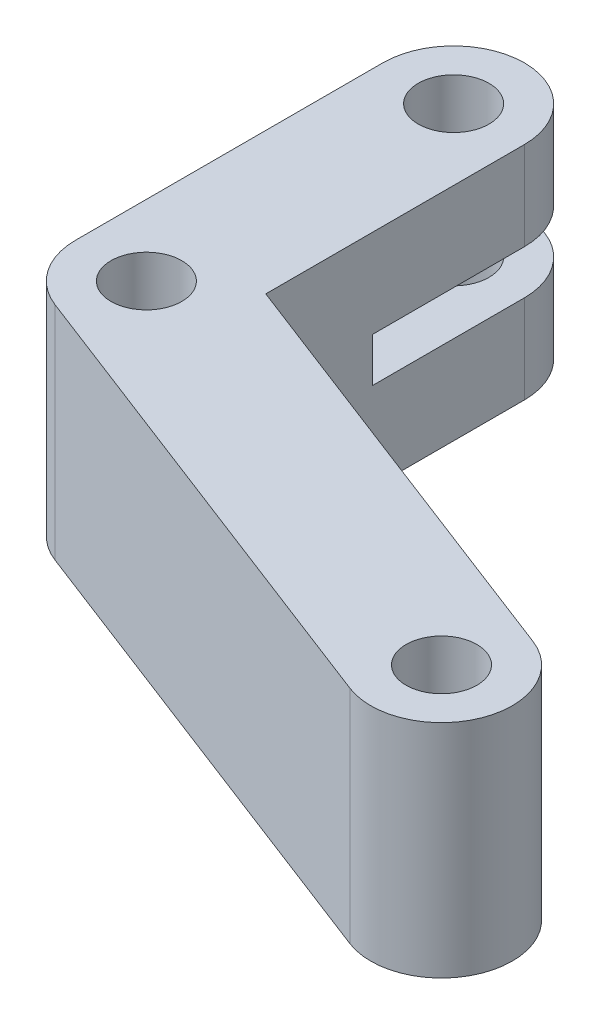
ISO-10303-21;
HEADER;
FILE_DESCRIPTION(('STEP AP214'),'2;1');
FILE_NAME('part.step','',(''),(''),'','','');
FILE_SCHEMA(('AUTOMOTIVE_DESIGN { 1 0 10303 214 1 1 1 1 }'));
ENDSEC;
DATA;
#1=APPLICATION_CONTEXT('core data for automotive mechanical design processes');
#2=APPLICATION_PROTOCOL_DEFINITION('international standard','automotive_design',2000,#1);
#3=PRODUCT_CONTEXT('',#1,'mechanical');
#4=PRODUCT('Part','Part','',(#3));
#5=PRODUCT_RELATED_PRODUCT_CATEGORY('part','',(#4));
#6=PRODUCT_DEFINITION_FORMATION('','',#4);
#7=PRODUCT_DEFINITION_CONTEXT('part definition',#1,'design');
#8=PRODUCT_DEFINITION('design','',#6,#7);
#9=PRODUCT_DEFINITION_SHAPE('','',#8);
#10=(LENGTH_UNIT() NAMED_UNIT(*) SI_UNIT(.MILLI.,.METRE.));
#11=(NAMED_UNIT(*) PLANE_ANGLE_UNIT() SI_UNIT($,.RADIAN.));
#12=(NAMED_UNIT(*) SI_UNIT($,.STERADIAN.) SOLID_ANGLE_UNIT());
#13=UNCERTAINTY_MEASURE_WITH_UNIT(LENGTH_MEASURE(1.E-05),#10,'distance_accuracy_value','');
#14=(GEOMETRIC_REPRESENTATION_CONTEXT(3) GLOBAL_UNCERTAINTY_ASSIGNED_CONTEXT((#13)) GLOBAL_UNIT_ASSIGNED_CONTEXT((#10,
#11,#12)) REPRESENTATION_CONTEXT('',''));
#15=CARTESIAN_POINT('',(0.,0.,0.));
#16=DIRECTION('',(0.,0.,1.));
#17=DIRECTION('',(1.,0.,0.));
#18=AXIS2_PLACEMENT_3D('',#15,#16,#17);
#19=CARTESIAN_POINT('',(0.,25.,-34.72));
#20=DIRECTION('',(0.,-1.,0.));
#21=DIRECTION('',(0.,0.,-1.));
#22=AXIS2_PLACEMENT_3D('',#19,#20,#21);
#23=CYLINDRICAL_SURFACE('',#22,8.);
#24=CARTESIAN_POINT('',(0.,10.,-34.72));
#25=DIRECTION('',(0.,-1.,0.));
#26=DIRECTION('',(0.,0.,-1.));
#27=AXIS2_PLACEMENT_3D('',#24,#25,#26);
#28=CIRCLE('',#27,8.);
#29=CARTESIAN_POINT('',(-8.,10.,-34.72));
#30=VERTEX_POINT('',#29);
#31=CARTESIAN_POINT('',(8.,10.,-34.72));
#32=VERTEX_POINT('',#31);
#33=EDGE_CURVE('E184',#30,#32,#28,.T.);
#34=ORIENTED_EDGE('',*,*,#33,.T.);
#35=DIRECTION('',(0.,-1.,0.));
#36=VECTOR('',#35,1.);
#37=CARTESIAN_POINT('',(8.,25.,-34.72));
#38=LINE('',#37,#36);
#39=CARTESIAN_POINT('',(8.,0.,-34.72));
#40=VERTEX_POINT('',#39);
#41=EDGE_CURVE('E96',#32,#40,#38,.T.);
#42=ORIENTED_EDGE('',*,*,#41,.T.);
#43=CARTESIAN_POINT('',(0.,0.,-34.72));
#44=DIRECTION('',(0.,1.,0.));
#45=DIRECTION('',(0.,0.,1.));
#46=AXIS2_PLACEMENT_3D('',#43,#44,#45);
#47=CIRCLE('',#46,8.);
#48=CARTESIAN_POINT('',(-8.00000000000001,0.,-34.72));
#49=VERTEX_POINT('',#48);
#50=EDGE_CURVE('E144',#40,#49,#47,.T.);
#51=ORIENTED_EDGE('',*,*,#50,.T.);
#52=DIRECTION('',(0.,-1.,0.));
#53=VECTOR('',#52,1.);
#54=CARTESIAN_POINT('',(-8.00000000000001,25.,-34.72));
#55=LINE('',#54,#53);
#56=EDGE_CURVE('E171',#30,#49,#55,.T.);
#57=ORIENTED_EDGE('',*,*,#56,.F.);
#58=EDGE_LOOP('',(#34,#42,#51,#57));
#59=FACE_BOUND('',#58,.T.);
#60=ADVANCED_FACE('F41',(#59),#23,.T.);
#61=CARTESIAN_POINT('',(0.,0.,-34.72));
#62=DIRECTION('',(0.,1.,0.));
#63=DIRECTION('',(0.,0.,1.));
#64=AXIS2_PLACEMENT_3D('',#61,#62,#63);
#65=CYLINDRICAL_SURFACE('',#64,4.);
#66=CARTESIAN_POINT('',(0.,10.,-34.72));
#67=DIRECTION('',(0.,-1.,0.));
#68=DIRECTION('',(0.,0.,-1.));
#69=AXIS2_PLACEMENT_3D('',#66,#67,#68);
#70=CIRCLE('',#69,4.);
#71=CARTESIAN_POINT('',(0.,10.,-38.72));
#72=VERTEX_POINT('',#71);
#73=EDGE_CURVE('E180',#72,#72,#70,.F.);
#74=ORIENTED_EDGE('',*,*,#73,.T.);
#75=EDGE_LOOP('',(#74));
#76=FACE_BOUND('',#75,.T.);
#77=CARTESIAN_POINT('',(0.,0.,-34.72));
#78=DIRECTION('',(0.,1.,0.));
#79=DIRECTION('',(0.,0.,1.));
#80=AXIS2_PLACEMENT_3D('',#77,#78,#79);
#81=CIRCLE('',#80,4.);
#82=CARTESIAN_POINT('',(0.,0.,-30.72));
#83=VERTEX_POINT('',#82);
#84=EDGE_CURVE('E146',#83,#83,#81,.T.);
#85=ORIENTED_EDGE('',*,*,#84,.F.);
#86=EDGE_LOOP('',(#85));
#87=FACE_BOUND('',#86,.T.);
#88=ADVANCED_FACE('F257',(#76,#87),#65,.F.);
#89=CARTESIAN_POINT('',(8.,25.,-34.72));
#90=VERTEX_POINT('',#89);
#91=CARTESIAN_POINT('',(8.,15.,-34.72));
#92=VERTEX_POINT('',#91);
#93=EDGE_CURVE('E159',#90,#92,#38,.T.);
#94=ORIENTED_EDGE('',*,*,#93,.T.);
#95=CARTESIAN_POINT('',(0.,15.,-34.72));
#96=DIRECTION('',(0.,1.,0.));
#97=DIRECTION('',(0.,0.,1.));
#98=AXIS2_PLACEMENT_3D('',#95,#96,#97);
#99=CIRCLE('',#98,8.);
#100=CARTESIAN_POINT('',(-8.,15.,-34.72));
#101=VERTEX_POINT('',#100);
#102=EDGE_CURVE('E57',#92,#101,#99,.T.);
#103=ORIENTED_EDGE('',*,*,#102,.T.);
#104=CARTESIAN_POINT('',(-8.00000000000001,25.,-34.72));
#105=VERTEX_POINT('',#104);
#106=EDGE_CURVE('E47',#105,#101,#55,.T.);
#107=ORIENTED_EDGE('',*,*,#106,.F.);
#108=CARTESIAN_POINT('',(0.,25.,-34.72));
#109=DIRECTION('',(0.,1.,0.));
#110=DIRECTION('',(0.,0.,1.));
#111=AXIS2_PLACEMENT_3D('',#108,#109,#110);
#112=CIRCLE('',#111,8.);
#113=EDGE_CURVE('E157',#90,#105,#112,.T.);
#114=ORIENTED_EDGE('',*,*,#113,.F.);
#115=EDGE_LOOP('',(#94,#103,#107,#114));
#116=FACE_BOUND('',#115,.T.);
#117=ADVANCED_FACE('F43',(#116),#23,.T.);
#118=CARTESIAN_POINT('',(-8.00000000000001,25.,-34.72));
#119=DIRECTION('',(1.,0.,0.));
#120=DIRECTION('',(0.,0.,-1.));
#121=AXIS2_PLACEMENT_3D('',#118,#119,#120);
#122=PLANE('',#121);
#123=DIRECTION('',(0.,-1.,0.));
#124=VECTOR('',#123,1.);
#125=CARTESIAN_POINT('',(-8.,25.,-17.57));
#126=LINE('',#125,#124);
#127=CARTESIAN_POINT('',(-8.,15.,-17.57));
#128=VERTEX_POINT('',#127);
#129=CARTESIAN_POINT('',(-8.,10.,-17.57));
#130=VERTEX_POINT('',#129);
#131=EDGE_CURVE('E197',#128,#130,#126,.T.);
#132=ORIENTED_EDGE('',*,*,#131,.T.);
#133=DIRECTION('',(0.,0.,-1.));
#134=VECTOR('',#133,1.);
#135=CARTESIAN_POINT('',(-8.00000000000001,10.,-34.72));
#136=LINE('',#135,#134);
#137=EDGE_CURVE('E192',#130,#30,#136,.T.);
#138=ORIENTED_EDGE('',*,*,#137,.T.);
#139=ORIENTED_EDGE('',*,*,#56,.T.);
#140=DIRECTION('',(0.,0.,1.));
#141=VECTOR('',#140,1.);
#142=CARTESIAN_POINT('',(-8.00000000000001,0.,-34.72));
#143=LINE('',#142,#141);
#144=CARTESIAN_POINT('',(-8.,0.,0.));
#145=VERTEX_POINT('',#144);
#146=EDGE_CURVE('E150',#49,#145,#143,.T.);
#147=ORIENTED_EDGE('',*,*,#146,.T.);
#148=DIRECTION('',(0.,-1.,0.));
#149=VECTOR('',#148,1.);
#150=CARTESIAN_POINT('',(-8.,25.,0.));
#151=LINE('',#150,#149);
#152=CARTESIAN_POINT('',(-8.,25.,0.));
#153=VERTEX_POINT('',#152);
#154=EDGE_CURVE('E169',#153,#145,#151,.T.);
#155=ORIENTED_EDGE('',*,*,#154,.F.);
#156=DIRECTION('',(0.,0.,1.));
#157=VECTOR('',#156,1.);
#158=CARTESIAN_POINT('',(-8.00000000000001,25.,-34.72));
#159=LINE('',#158,#157);
#160=EDGE_CURVE('E104',#105,#153,#159,.T.);
#161=ORIENTED_EDGE('',*,*,#160,.F.);
#162=ORIENTED_EDGE('',*,*,#106,.T.);
#163=DIRECTION('',(0.,0.,1.));
#164=VECTOR('',#163,1.);
#165=CARTESIAN_POINT('',(-8.00000000000001,15.,-34.72));
#166=LINE('',#165,#164);
#167=EDGE_CURVE('E179',#101,#128,#166,.T.);
#168=ORIENTED_EDGE('',*,*,#167,.T.);
#169=EDGE_LOOP('',(#132,#138,#139,#147,#155,#161,#162,#168));
#170=FACE_BOUND('',#169,.T.);
#171=ADVANCED_FACE('F240',(#170),#122,.F.);
#172=CARTESIAN_POINT('',(0.,25.,0.));
#173=DIRECTION('',(0.,-1.,0.));
#174=DIRECTION('',(0.,0.,-1.));
#175=AXIS2_PLACEMENT_3D('',#172,#173,#174);
#176=CYLINDRICAL_SURFACE('',#175,8.);
#177=CARTESIAN_POINT('',(0.,0.,0.));
#178=DIRECTION('',(0.,1.,0.));
#179=DIRECTION('',(0.,0.,1.));
#180=AXIS2_PLACEMENT_3D('',#177,#178,#179);
#181=CIRCLE('',#180,8.);
#182=CARTESIAN_POINT('',(-2.87524489022323,0.,7.46545154838239));
#183=VERTEX_POINT('',#182);
#184=EDGE_CURVE('E147',#145,#183,#181,.T.);
#185=ORIENTED_EDGE('',*,*,#184,.T.);
#186=DIRECTION('',(0.,-1.,0.));
#187=VECTOR('',#186,1.);
#188=CARTESIAN_POINT('',(-2.87524489022323,25.,7.46545154838239));
#189=LINE('',#188,#187);
#190=CARTESIAN_POINT('',(-2.87524489022323,25.,7.46545154838239));
#191=VERTEX_POINT('',#190);
#192=EDGE_CURVE('E164',#191,#183,#189,.T.);
#193=ORIENTED_EDGE('',*,*,#192,.F.);
#194=CARTESIAN_POINT('',(0.,25.,0.));
#195=DIRECTION('',(0.,1.,0.));
#196=DIRECTION('',(0.,0.,1.));
#197=AXIS2_PLACEMENT_3D('',#194,#195,#196);
#198=CIRCLE('',#197,8.);
#199=EDGE_CURVE('E217',#153,#191,#198,.T.);
#200=ORIENTED_EDGE('',*,*,#199,.F.);
#201=ORIENTED_EDGE('',*,*,#154,.T.);
#202=EDGE_LOOP('',(#185,#193,#200,#201));
#203=FACE_BOUND('',#202,.T.);
#204=ADVANCED_FACE('F225',(#203),#176,.T.);
#205=CARTESIAN_POINT('',(-2.87524489022323,25.,7.46545154838239));
#206=DIRECTION('',(0.359405611277904,0.,-0.9331814435478));
#207=DIRECTION('',(-0.9331814435478,0.,-0.359405611277904));
#208=AXIS2_PLACEMENT_3D('',#205,#206,#207);
#209=PLANE('',#208);
#210=DIRECTION('',(0.9331814435478,0.,0.359405611277904));
#211=VECTOR('',#210,1.);
#212=CARTESIAN_POINT('',(-2.87524489022323,0.,7.46545154838239));
#213=LINE('',#212,#211);
#214=CARTESIAN_POINT('',(51.3647551097768,0.,28.3554515483825));
#215=VERTEX_POINT('',#214);
#216=EDGE_CURVE('E155',#183,#215,#213,.T.);
#217=ORIENTED_EDGE('',*,*,#216,.T.);
#218=DIRECTION('',(0.,-1.,0.));
#219=VECTOR('',#218,1.);
#220=CARTESIAN_POINT('',(51.3647551097768,25.,28.3554515483825));
#221=LINE('',#220,#219);
#222=CARTESIAN_POINT('',(51.3647551097768,25.,28.3554515483825));
#223=VERTEX_POINT('',#222);
#224=EDGE_CURVE('E136',#223,#215,#221,.T.);
#225=ORIENTED_EDGE('',*,*,#224,.F.);
#226=DIRECTION('',(0.9331814435478,0.,0.359405611277904));
#227=VECTOR('',#226,1.);
#228=CARTESIAN_POINT('',(-2.87524489022323,25.,7.46545154838239));
#229=LINE('',#228,#227);
#230=EDGE_CURVE('E122',#191,#223,#229,.T.);
#231=ORIENTED_EDGE('',*,*,#230,.F.);
#232=ORIENTED_EDGE('',*,*,#192,.T.);
#233=EDGE_LOOP('',(#217,#225,#231,#232));
#234=FACE_BOUND('',#233,.T.);
#235=ADVANCED_FACE('F226',(#234),#209,.F.);
#236=CARTESIAN_POINT('',(54.24,25.,20.89));
#237=DIRECTION('',(0.,-1.,0.));
#238=DIRECTION('',(0.,0.,-1.));
#239=AXIS2_PLACEMENT_3D('',#236,#237,#238);
#240=CYLINDRICAL_SURFACE('',#239,8.00000000000006);
#241=CARTESIAN_POINT('',(54.24,0.,20.89));
#242=DIRECTION('',(0.,1.,0.));
#243=DIRECTION('',(0.,0.,1.));
#244=AXIS2_PLACEMENT_3D('',#241,#242,#243);
#245=CIRCLE('',#244,8.00000000000006);
#246=CARTESIAN_POINT('',(57.1152448902233,0.,13.4245484516175));
#247=VERTEX_POINT('',#246);
#248=EDGE_CURVE('E134',#215,#247,#245,.T.);
#249=ORIENTED_EDGE('',*,*,#248,.T.);
#250=DIRECTION('',(0.,-1.,0.));
#251=VECTOR('',#250,1.);
#252=CARTESIAN_POINT('',(57.1152448902233,25.,13.4245484516175));
#253=LINE('',#252,#251);
#254=CARTESIAN_POINT('',(57.1152448902233,25.,13.4245484516175));
#255=VERTEX_POINT('',#254);
#256=EDGE_CURVE('E128',#255,#247,#253,.T.);
#257=ORIENTED_EDGE('',*,*,#256,.F.);
#258=CARTESIAN_POINT('',(54.24,25.,20.89));
#259=DIRECTION('',(0.,1.,0.));
#260=DIRECTION('',(0.,0.,1.));
#261=AXIS2_PLACEMENT_3D('',#258,#259,#260);
#262=CIRCLE('',#261,8.00000000000006);
#263=EDGE_CURVE('E117',#223,#255,#262,.T.);
#264=ORIENTED_EDGE('',*,*,#263,.F.);
#265=ORIENTED_EDGE('',*,*,#224,.T.);
#266=EDGE_LOOP('',(#249,#257,#264,#265));
#267=FACE_BOUND('',#266,.T.);
#268=ADVANCED_FACE('F131',(#267),#240,.T.);
#269=CARTESIAN_POINT('',(8.,25.,-5.49170276071211));
#270=DIRECTION('',(-0.359405611277902,0.,0.933181443547801));
#271=DIRECTION('',(0.933181443547801,0.,0.359405611277902));
#272=AXIS2_PLACEMENT_3D('',#269,#270,#271);
#273=PLANE('',#272);
#274=DIRECTION('',(-0.933181443547801,0.,-0.359405611277902));
#275=VECTOR('',#274,1.);
#276=CARTESIAN_POINT('',(8.,0.,-5.49170276071211));
#277=LINE('',#276,#275);
#278=CARTESIAN_POINT('',(8.,0.,-5.49170276071211));
#279=VERTEX_POINT('',#278);
#280=EDGE_CURVE('E154',#247,#279,#277,.T.);
#281=ORIENTED_EDGE('',*,*,#280,.T.);
#282=DIRECTION('',(0.,-1.,0.));
#283=VECTOR('',#282,1.);
#284=CARTESIAN_POINT('',(8.,25.,-5.49170276071211));
#285=LINE('',#284,#283);
#286=CARTESIAN_POINT('',(8.,25.,-5.49170276071211));
#287=VERTEX_POINT('',#286);
#288=EDGE_CURVE('E140',#287,#279,#285,.T.);
#289=ORIENTED_EDGE('',*,*,#288,.F.);
#290=DIRECTION('',(-0.933181443547801,0.,-0.359405611277902));
#291=VECTOR('',#290,1.);
#292=CARTESIAN_POINT('',(8.,25.,-5.49170276071211));
#293=LINE('',#292,#291);
#294=EDGE_CURVE('E121',#255,#287,#293,.T.);
#295=ORIENTED_EDGE('',*,*,#294,.F.);
#296=ORIENTED_EDGE('',*,*,#256,.T.);
#297=EDGE_LOOP('',(#281,#289,#295,#296));
#298=FACE_BOUND('',#297,.T.);
#299=ADVANCED_FACE('F137',(#298),#273,.F.);
#300=CARTESIAN_POINT('',(8.,25.,-34.72));
#301=DIRECTION('',(-1.,0.,0.));
#302=DIRECTION('',(0.,0.,1.));
#303=AXIS2_PLACEMENT_3D('',#300,#301,#302);
#304=PLANE('',#303);
#305=ORIENTED_EDGE('',*,*,#41,.F.);
#306=DIRECTION('',(0.,0.,1.));
#307=VECTOR('',#306,1.);
#308=CARTESIAN_POINT('',(8.,10.,-34.72));
#309=LINE('',#308,#307);
#310=CARTESIAN_POINT('',(8.,10.,-17.57));
#311=VERTEX_POINT('',#310);
#312=EDGE_CURVE('E177',#32,#311,#309,.T.);
#313=ORIENTED_EDGE('',*,*,#312,.T.);
#314=DIRECTION('',(0.,1.,0.));
#315=VECTOR('',#314,1.);
#316=CARTESIAN_POINT('',(8.,25.,-17.57));
#317=LINE('',#316,#315);
#318=CARTESIAN_POINT('',(8.,15.,-17.57));
#319=VERTEX_POINT('',#318);
#320=EDGE_CURVE('E11',#311,#319,#317,.T.);
#321=ORIENTED_EDGE('',*,*,#320,.T.);
#322=DIRECTION('',(0.,0.,-1.));
#323=VECTOR('',#322,1.);
#324=CARTESIAN_POINT('',(8.,15.,-34.72));
#325=LINE('',#324,#323);
#326=EDGE_CURVE('E175',#319,#92,#325,.T.);
#327=ORIENTED_EDGE('',*,*,#326,.T.);
#328=ORIENTED_EDGE('',*,*,#93,.F.);
#329=DIRECTION('',(0.,0.,-1.));
#330=VECTOR('',#329,1.);
#331=CARTESIAN_POINT('',(8.,25.,-34.72));
#332=LINE('',#331,#330);
#333=EDGE_CURVE('E65',#287,#90,#332,.T.);
#334=ORIENTED_EDGE('',*,*,#333,.F.);
#335=ORIENTED_EDGE('',*,*,#288,.T.);
#336=DIRECTION('',(0.,0.,-1.));
#337=VECTOR('',#336,1.);
#338=CARTESIAN_POINT('',(8.,0.,-34.72));
#339=LINE('',#338,#337);
#340=EDGE_CURVE('E160',#279,#40,#339,.T.);
#341=ORIENTED_EDGE('',*,*,#340,.T.);
#342=EDGE_LOOP('',(#305,#313,#321,#327,#328,#334,#335,#341));
#343=FACE_BOUND('',#342,.T.);
#344=ADVANCED_FACE('F235',(#343),#304,.F.);
#345=CARTESIAN_POINT('',(0.,25.,-34.72));
#346=DIRECTION('',(0.,1.,0.));
#347=DIRECTION('',(0.,0.,1.));
#348=AXIS2_PLACEMENT_3D('',#345,#346,#347);
#349=PLANE('',#348);
#350=CARTESIAN_POINT('',(0.,25.,-34.72));
#351=DIRECTION('',(0.,1.,0.));
#352=DIRECTION('',(0.,0.,1.));
#353=AXIS2_PLACEMENT_3D('',#350,#351,#352);
#354=CIRCLE('',#353,4.);
#355=CARTESIAN_POINT('',(0.,25.,-30.72));
#356=VERTEX_POINT('',#355);
#357=EDGE_CURVE('E205',#356,#356,#354,.T.);
#358=ORIENTED_EDGE('',*,*,#357,.F.);
#359=EDGE_LOOP('',(#358));
#360=FACE_BOUND('',#359,.T.);
#361=CARTESIAN_POINT('',(54.24,25.,20.89));
#362=DIRECTION('',(0.,1.,0.));
#363=DIRECTION('',(0.,0.,1.));
#364=AXIS2_PLACEMENT_3D('',#361,#362,#363);
#365=CIRCLE('',#364,4.00000000000001);
#366=CARTESIAN_POINT('',(54.24,25.,24.89));
#367=VERTEX_POINT('',#366);
#368=EDGE_CURVE('E202',#367,#367,#365,.T.);
#369=ORIENTED_EDGE('',*,*,#368,.F.);
#370=EDGE_LOOP('',(#369));
#371=FACE_BOUND('',#370,.T.);
#372=CARTESIAN_POINT('',(0.,25.,0.));
#373=DIRECTION('',(0.,1.,0.));
#374=DIRECTION('',(0.,0.,1.));
#375=AXIS2_PLACEMENT_3D('',#372,#373,#374);
#376=CIRCLE('',#375,4.);
#377=CARTESIAN_POINT('',(0.,25.,4.));
#378=VERTEX_POINT('',#377);
#379=EDGE_CURVE('E211',#378,#378,#376,.T.);
#380=ORIENTED_EDGE('',*,*,#379,.F.);
#381=EDGE_LOOP('',(#380));
#382=FACE_BOUND('',#381,.T.);
#383=ORIENTED_EDGE('',*,*,#113,.T.);
#384=ORIENTED_EDGE('',*,*,#160,.T.);
#385=ORIENTED_EDGE('',*,*,#199,.T.);
#386=ORIENTED_EDGE('',*,*,#230,.T.);
#387=ORIENTED_EDGE('',*,*,#263,.T.);
#388=ORIENTED_EDGE('',*,*,#294,.T.);
#389=ORIENTED_EDGE('',*,*,#333,.T.);
#390=EDGE_LOOP('',(#383,#384,#385,#386,#387,#388,#389));
#391=FACE_BOUND('',#390,.T.);
#392=ADVANCED_FACE('F118',(#360,#371,#382,#391),#349,.T.);
#393=CARTESIAN_POINT('',(0.,0.,-34.72));
#394=DIRECTION('',(0.,1.,0.));
#395=DIRECTION('',(0.,0.,1.));
#396=AXIS2_PLACEMENT_3D('',#393,#394,#395);
#397=PLANE('',#396);
#398=ORIENTED_EDGE('',*,*,#84,.T.);
#399=EDGE_LOOP('',(#398));
#400=FACE_BOUND('',#399,.T.);
#401=CARTESIAN_POINT('',(54.24,0.,20.89));
#402=DIRECTION('',(0.,1.,0.));
#403=DIRECTION('',(0.,0.,1.));
#404=AXIS2_PLACEMENT_3D('',#401,#402,#403);
#405=CIRCLE('',#404,4.00000000000001);
#406=CARTESIAN_POINT('',(54.24,0.,24.89));
#407=VERTEX_POINT('',#406);
#408=EDGE_CURVE('E208',#407,#407,#405,.T.);
#409=ORIENTED_EDGE('',*,*,#408,.T.);
#410=EDGE_LOOP('',(#409));
#411=FACE_BOUND('',#410,.T.);
#412=CARTESIAN_POINT('',(0.,0.,0.));
#413=DIRECTION('',(0.,1.,0.));
#414=DIRECTION('',(0.,0.,1.));
#415=AXIS2_PLACEMENT_3D('',#412,#413,#414);
#416=CIRCLE('',#415,4.);
#417=CARTESIAN_POINT('',(0.,0.,4.));
#418=VERTEX_POINT('',#417);
#419=EDGE_CURVE('E200',#418,#418,#416,.T.);
#420=ORIENTED_EDGE('',*,*,#419,.T.);
#421=EDGE_LOOP('',(#420));
#422=FACE_BOUND('',#421,.T.);
#423=ORIENTED_EDGE('',*,*,#50,.F.);
#424=ORIENTED_EDGE('',*,*,#340,.F.);
#425=ORIENTED_EDGE('',*,*,#280,.F.);
#426=ORIENTED_EDGE('',*,*,#248,.F.);
#427=ORIENTED_EDGE('',*,*,#216,.F.);
#428=ORIENTED_EDGE('',*,*,#184,.F.);
#429=ORIENTED_EDGE('',*,*,#146,.F.);
#430=EDGE_LOOP('',(#423,#424,#425,#426,#427,#428,#429));
#431=FACE_BOUND('',#430,.T.);
#432=ADVANCED_FACE('F228',(#400,#411,#422,#431),#397,.F.);
#433=CARTESIAN_POINT('',(0.,0.,0.));
#434=DIRECTION('',(0.,1.,0.));
#435=DIRECTION('',(0.,0.,1.));
#436=AXIS2_PLACEMENT_3D('',#433,#434,#435);
#437=CYLINDRICAL_SURFACE('',#436,4.);
#438=ORIENTED_EDGE('',*,*,#419,.F.);
#439=EDGE_LOOP('',(#438));
#440=FACE_BOUND('',#439,.T.);
#441=ORIENTED_EDGE('',*,*,#379,.T.);
#442=EDGE_LOOP('',(#441));
#443=FACE_BOUND('',#442,.T.);
#444=ADVANCED_FACE('F286',(#440,#443),#437,.F.);
#445=CARTESIAN_POINT('',(54.24,0.,20.89));
#446=DIRECTION('',(0.,1.,0.));
#447=DIRECTION('',(0.,0.,1.));
#448=AXIS2_PLACEMENT_3D('',#445,#446,#447);
#449=CYLINDRICAL_SURFACE('',#448,4.00000000000001);
#450=ORIENTED_EDGE('',*,*,#408,.F.);
#451=EDGE_LOOP('',(#450));
#452=FACE_BOUND('',#451,.T.);
#453=ORIENTED_EDGE('',*,*,#368,.T.);
#454=EDGE_LOOP('',(#453));
#455=FACE_BOUND('',#454,.T.);
#456=ADVANCED_FACE('F291',(#452,#455),#449,.F.);
#457=CARTESIAN_POINT('',(0.,15.,-34.72));
#458=DIRECTION('',(0.,1.,0.));
#459=DIRECTION('',(0.,0.,1.));
#460=AXIS2_PLACEMENT_3D('',#457,#458,#459);
#461=CIRCLE('',#460,4.);
#462=CARTESIAN_POINT('',(0.,15.,-30.72));
#463=VERTEX_POINT('',#462);
#464=EDGE_CURVE('E174',#463,#463,#461,.F.);
#465=ORIENTED_EDGE('',*,*,#464,.T.);
#466=EDGE_LOOP('',(#465));
#467=FACE_BOUND('',#466,.T.);
#468=ORIENTED_EDGE('',*,*,#357,.T.);
#469=EDGE_LOOP('',(#468));
#470=FACE_BOUND('',#469,.T.);
#471=ADVANCED_FACE('F266',(#467,#470),#65,.F.);
#472=CARTESIAN_POINT('',(-12.5,15.,-17.57));
#473=DIRECTION('',(0.,0.,1.));
#474=DIRECTION('',(1.,0.,0.));
#475=AXIS2_PLACEMENT_3D('',#472,#473,#474);
#476=PLANE('',#475);
#477=DIRECTION('',(1.,0.,0.));
#478=VECTOR('',#477,1.);
#479=CARTESIAN_POINT('',(-12.5,15.,-17.57));
#480=LINE('',#479,#478);
#481=EDGE_CURVE('E406',#128,#319,#480,.T.);
#482=ORIENTED_EDGE('',*,*,#481,.T.);
#483=ORIENTED_EDGE('',*,*,#320,.F.);
#484=DIRECTION('',(1.,0.,0.));
#485=VECTOR('',#484,1.);
#486=CARTESIAN_POINT('',(-12.5,10.,-17.57));
#487=LINE('',#486,#485);
#488=EDGE_CURVE('E176',#130,#311,#487,.T.);
#489=ORIENTED_EDGE('',*,*,#488,.F.);
#490=ORIENTED_EDGE('',*,*,#131,.F.);
#491=EDGE_LOOP('',(#482,#483,#489,#490));
#492=FACE_BOUND('',#491,.T.);
#493=ADVANCED_FACE('F299',(#492),#476,.F.);
#494=CARTESIAN_POINT('',(-12.5,10.,-42.72));
#495=DIRECTION('',(0.,-1.,0.));
#496=DIRECTION('',(0.,0.,-1.));
#497=AXIS2_PLACEMENT_3D('',#494,#495,#496);
#498=PLANE('',#497);
#499=ORIENTED_EDGE('',*,*,#73,.F.);
#500=EDGE_LOOP('',(#499));
#501=FACE_BOUND('',#500,.T.);
#502=ORIENTED_EDGE('',*,*,#488,.T.);
#503=ORIENTED_EDGE('',*,*,#312,.F.);
#504=ORIENTED_EDGE('',*,*,#33,.F.);
#505=ORIENTED_EDGE('',*,*,#137,.F.);
#506=EDGE_LOOP('',(#502,#503,#504,#505));
#507=FACE_BOUND('',#506,.T.);
#508=ADVANCED_FACE('F254',(#501,#507),#498,.F.);
#509=CARTESIAN_POINT('',(-12.5,15.,-42.72));
#510=DIRECTION('',(0.,1.,0.));
#511=DIRECTION('',(0.,0.,1.));
#512=AXIS2_PLACEMENT_3D('',#509,#510,#511);
#513=PLANE('',#512);
#514=ORIENTED_EDGE('',*,*,#464,.F.);
#515=EDGE_LOOP('',(#514));
#516=FACE_BOUND('',#515,.T.);
#517=ORIENTED_EDGE('',*,*,#102,.F.);
#518=ORIENTED_EDGE('',*,*,#326,.F.);
#519=ORIENTED_EDGE('',*,*,#481,.F.);
#520=ORIENTED_EDGE('',*,*,#167,.F.);
#521=EDGE_LOOP('',(#517,#518,#519,#520));
#522=FACE_BOUND('',#521,.T.);
#523=ADVANCED_FACE('F300',(#516,#522),#513,.F.);
#524=CLOSED_SHELL('',(#60,#88,#117,#171,#204,#235,#268,#299,#344,#392,#432,#444,#456,#471,#493,
#508,#523));
#525=MANIFOLD_SOLID_BREP('B2',#524);
#526=ADVANCED_BREP_SHAPE_REPRESENTATION('',(#18,#525),#14);
#527=SHAPE_DEFINITION_REPRESENTATION(#9,#526);
ENDSEC;
END-ISO-10303-21;
